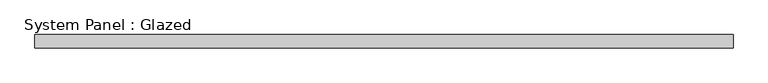
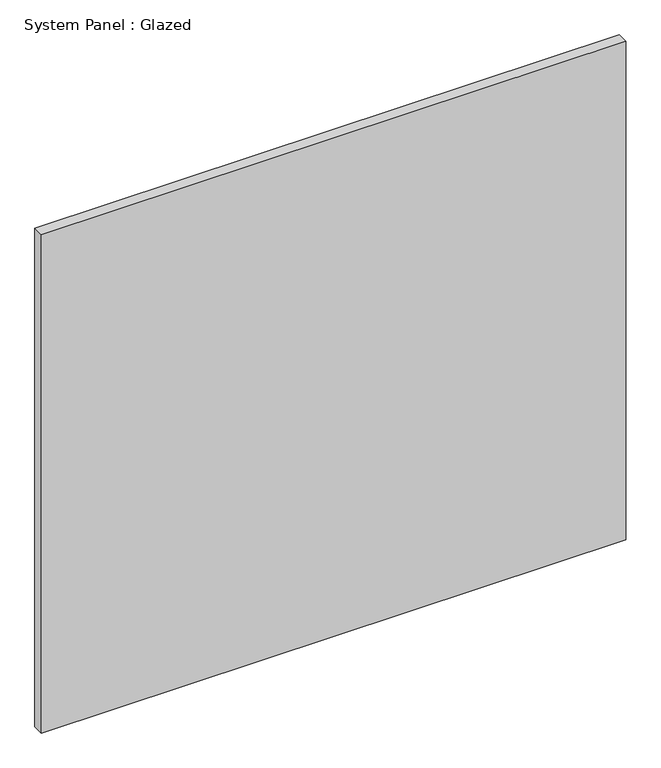
"""IFC4 building model written with IfcOpenShell, lengths in millimetres: plate geometry, System Panel : Glazed."""

from ifc_helpers import new_model, si_unit, origin, origin_with_axes, place, context, project, spatial, polyline, outline, extrude, source, transform, mapped, element, save


def system_panel_glazed_07392c36(model_context):
    return source(origin(), model_context, "Body", "SweptSolid", [
        extrude(outline(polyline([(676.275, 19.05), (-676.275, 19.05), (-676.275, 44.45), (676.275, 44.45), (676.275, 19.05)])), origin_with_axes(), (0.0, 0.0, 1.0), 1219.2),
    ])


if __name__ == "__main__":
    model = new_model("IFC4")
    model_context = context("Model", 3, world=origin())
    ifc_project = project(units=[si_unit("LENGTHUNIT", "METRE", prefix="MILLI")], contexts=[model_context])
    site = spatial("IfcSite", under=ifc_project)
    building = spatial("IfcBuilding", under=site)
    placement = place(None, origin())
    system_panel_glazed_shape = system_panel_glazed_07392c36(model_context)
    element("IfcPlate", 1, ObjectType="System Panel : Glazed", at=placement, inside=building, context=model_context, shape_type="MappedRepresentation", body=[
        mapped(system_panel_glazed_shape, transform((0.0, 0.0, 0.0), x_axis=(1.0, 0.0, 0.0), y_axis=(0.0, 1.0, 0.0), z_axis=(0.0, 0.0, 1.0))),
    ])
    save(model, "model.ifc")

# Revit data of these elements
# Type "System Panel : Glazed"
#   Construction Type Id = "GSP4R"
#   Analytic Construction = "1/8 in Pilkington single glazing"
#   Visual Light Transmittance = 0.9
#   Solar Heat Gain Coefficient = 0.86
#   Heat Transfer Coefficient (U) = 1.18115 BTU/(h·ft²·°F)
# Element 1 (IfcPlate, "System Panel : Glazed")
#   Materials on its faces: "Glass"
# Materials
#   "Glass": class "Glass", colour RGB 0 128 192, transparency 0.75, Description = "Soda Lime Glass", Cost = 0
